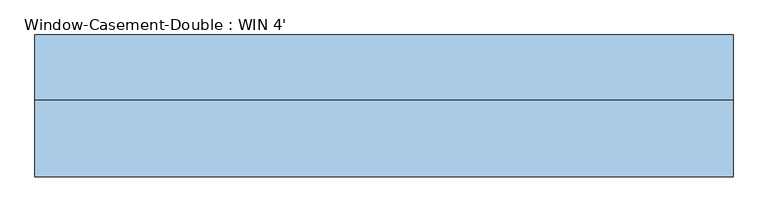
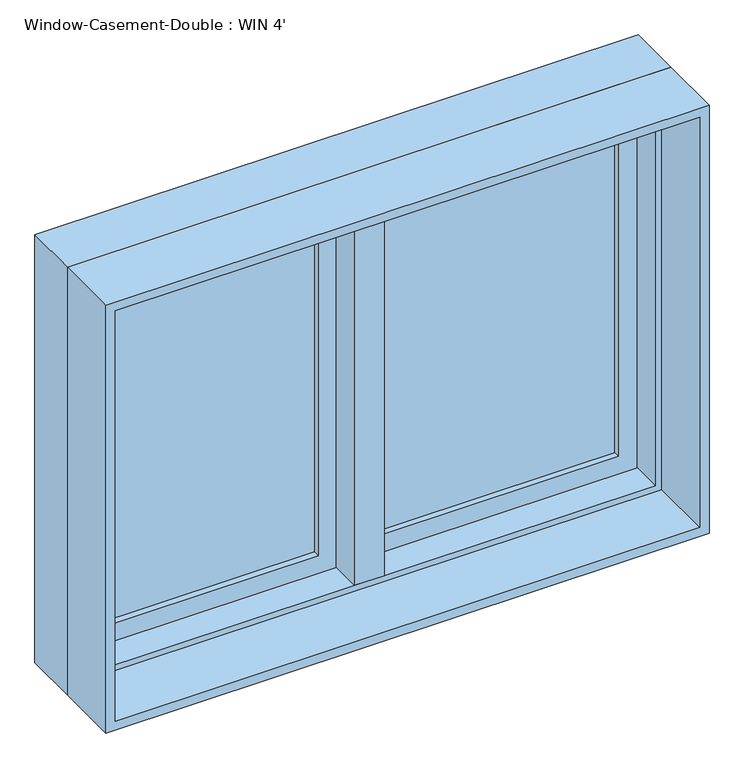
"""IFC4 building model written with IfcOpenShell, lengths in millimetres: window geometry, Window-Casement-Double : WIN 4'."""

from ifc_helpers import new_model, si_unit, frame, origin, place, context, project, spatial, polyline, outline, extrude, faceted_brep, source, transform, mapped, element, save


def window_casement_double_win_4_c19c33cb(model_context):
    return source(origin(), model_context, "Body", "SolidModel", [
        faceted_brep([(9.525, 133.35, 1816.1), (-9.525, 133.35, 1816.1), (-9.525, 82.55, 1816.1), (9.525, 82.55, 1816.1), (9.525, 133.35, 927.1), (9.525, 82.55, 927.1), (-9.525, 82.55, 927.1), (-9.525, 133.35, 927.1), (-9.525, 82.55, 946.15), (-9.525, 82.55, 1797.05), (-30.1625, 82.55, 946.15), (-30.1625, 82.55, 1797.05), (-30.1625, 19.05, 946.15), (-30.1625, 19.05, 1797.05), (30.1625, 19.05, 946.15), (30.1625, 19.05, 1797.05), (30.1625, 82.55, 946.15), (30.1625, 82.55, 1797.05), (9.525, 82.55, 946.15), (9.525, 82.55, 1797.05)], [[[0, 1, 2, 3]], [[4, 5, 6, 7]], [[1, 0, 4, 7]], [[2, 1, 7, 6, 8, 9]], [[9, 8, 10, 11]], [[11, 10, 12, 13]], [[13, 12, 14, 15]], [[15, 14, 16, 17]], [[17, 16, 18, 19]], [[0, 3, 19, 18, 5, 4]], [[18, 8, 6, 5]], [[9, 19, 3, 2]], [[8, 18, 16, 14, 12, 10]], [[19, 9, 11, 13, 15, 17]]]),
        extrude(outline(polyline([(-66.675, 114.3), (-66.675, 107.95), (-539.75, 107.95), (-539.75, 114.3), (-66.675, 114.3)])), frame((0.0, 0.0, 984.25), z_axis=(0.0, 0.0, 1.0), x_axis=(1.0, 0.0, 0.0)), (0.0, 0.0, 1.0), 774.7),
        extrude(outline(polyline([(-539.75, 95.25), (-539.75, 101.6), (-66.675, 101.6), (-66.675, 95.25), (-539.75, 95.25)])), frame((0.0, 0.0, 984.25), z_axis=(0.0, 0.0, 1.0), x_axis=(1.0, 0.0, 0.0)), (0.0, 0.0, 1.0), 774.7),
        extrude(outline(polyline([(539.75, 114.3), (539.75, 107.95), (66.675, 107.95), (66.675, 114.3), (539.75, 114.3)])), frame((0.0, 0.0, 984.25), z_axis=(0.0, 0.0, 1.0), x_axis=(1.0, 0.0, 0.0)), (0.0, 0.0, 1.0), 774.7),
        extrude(outline(polyline([(66.675, 95.25), (66.675, 101.6), (539.75, 101.6), (539.75, 95.25), (66.675, 95.25)])), frame((0.0, 0.0, 984.25), z_axis=(0.0, 0.0, 1.0), x_axis=(1.0, 0.0, 0.0)), (0.0, 0.0, 1.0), 774.7),
        extrude(outline(polyline([(1816.1, -596.9), (927.1, -596.9), (927.1, -9.525), (1816.1, -9.525), (1816.1, -596.9)]), holes=[polyline([(1758.95, -66.675), (984.25, -66.675), (984.25, -539.75), (1758.95, -539.75), (1758.95, -66.675)])]), frame((0.0, 82.55, 0.0), z_axis=(0.0, 1.0, 0.0), x_axis=(0.0, 0.0, 1.0)), (0.0, 0.0, 1.0), 44.45),
        extrude(outline(polyline([(927.1, 596.9), (1816.1, 596.9), (1816.1, 9.525), (927.1, 9.525), (927.1, 596.9)]), holes=[polyline([(984.25, 66.675), (1758.95, 66.675), (1758.95, 539.75), (984.25, 539.75), (984.25, 66.675)])]), frame((0.0, 82.55, 0.0), z_axis=(0.0, 1.0, 0.0), x_axis=(0.0, 0.0, 1.0)), (0.0, 0.0, 1.0), 44.45),
        extrude(outline(polyline([(1828.8, -609.6), (914.4, -609.6), (914.4, 609.6), (1828.8, 609.6), (1828.8, -609.6)]), holes=[polyline([(1809.75, 590.55), (933.45, 590.55), (933.45, -590.55), (1809.75, -590.55), (1809.75, 590.55)])]), frame((0.0, -114.3, 0.0), z_axis=(0.0, 1.0, 0.0), x_axis=(0.0, 0.0, 1.0)), (0.0, 0.0, 1.0), 133.35),
        faceted_brep([(577.85, 82.55, 1797.05), (577.85, 19.05, 1797.05), (-577.85, 19.05, 1797.05), (-577.85, 82.55, 1797.05), (596.9, 133.35, 1816.1), (596.9, 82.55, 1816.1), (-596.9, 82.55, 1816.1), (-596.9, 133.35, 1816.1), (609.6, 19.05, 1828.8), (609.6, 133.35, 1828.8), (-609.6, 133.35, 1828.8), (-609.6, 19.05, 1828.8), (-577.85, 19.05, 946.15), (-577.85, 82.55, 946.15), (-596.9, 82.55, 927.1), (-596.9, 133.35, 927.1), (-609.6, 133.35, 914.4), (-609.6, 19.05, 914.4), (577.85, 19.05, 946.15), (577.85, 82.55, 946.15), (596.9, 82.55, 927.1), (596.9, 133.35, 927.1), (609.6, 133.35, 914.4), (609.6, 19.05, 914.4)], [[[0, 1, 2, 3]], [[4, 5, 6, 7]], [[8, 9, 10, 11]], [[3, 2, 12, 13]], [[7, 6, 14, 15]], [[11, 10, 16, 17]], [[13, 12, 18, 19]], [[15, 14, 20, 21]], [[17, 16, 22, 23]], [[11, 17, 23, 8], [1, 18, 12, 2]], [[19, 18, 1, 0]], [[5, 20, 14, 6], [3, 13, 19, 0]], [[21, 20, 5, 4]], [[23, 22, 9, 8]], [[9, 22, 16, 10], [7, 15, 21, 4]]]),
    ])


if __name__ == "__main__":
    model = new_model("IFC4")
    model_context = context("Model", 3, world=origin())
    ifc_project = project(units=[si_unit("LENGTHUNIT", "METRE", prefix="MILLI")], contexts=[model_context])
    site = spatial("IfcSite", under=ifc_project)
    building = spatial("IfcBuilding", under=site)
    placement = place(None, origin())
    window_casement_double_win_4_shape = window_casement_double_win_4_c19c33cb(model_context)
    element("IfcWindow", 1, ObjectType="Window-Casement-Double : WIN 4'", at=placement, inside=building, context=model_context, shape_type="MappedRepresentation", body=[
        mapped(window_casement_double_win_4_shape, transform((0.0, 0.0, 0.0), x_axis=(1.0, 0.0, 0.0), y_axis=(0.0, 1.0, 0.0), z_axis=(0.0, 0.0, 1.0))),
    ])
    save(model, "model.ifc")

# Revit data of these elements
# Type "Window-Casement-Double : WIN 4'"
#   Type Mark = "18"
#   Fire Rating = "0.5h"
#   Assembly Code = "B2020100"
#   Analytic Construction = "Double glazing - domestic"
#   Frame Extension [instance default] = 0' - 0 1/4"
#   Window Inset [instance default] = 0' - 0"
#   Wall Thickness [instance default] = 0' - 6"
#   Interior Wall Closure [instance default] = 0' - 2 1/4"
#   Half Width = 2' - 0"
#   Visual Light Transmittance = 0.81
#   Thermal Resistance (R) = 1.8146 (h·ft²·°F)/BTU
#   Solar Heat Gain Coefficient = 0.76
#   Rough Width = 4' - 0 1/2"
#   Rough Height = 3' - 0 1/2"
#   Height = 3' - 0"
#   Heat Transfer Coefficient (U) = 0.5511 BTU/(h·ft²·°F)
#   Exterior Wall Closure [instance default] = 0' - 1 1/4"
#   Extension Jamb [instance default] = 0' - 2 1/4"
#   Default Sill Height = 3' - 0"
#   Width = 4' - 0"
#   Muntin Visibility = yes
#   Interior Trim Visibility [instance default] = yes
#   Exterior Trim Visibility [instance default] = yes
#   Extension Jamb Visibility [instance default] = yes
#   Interior Trim Material = Wood - Stained
#   Muntin Pattern = Muntin Pattern_2x2 : Muntin Pattern_2x2
#   Interior Trim = Trim-Window-Interior-Flat : Picture Frame
#   Interior Frame Material = Wood - Stained
#   Glass Panel Material = Glass
#   Exterior Trim Material = Clad - White
#   Exterior Trim = Trim-Window-Exterior-Flat : with Sill
#   Exterior Frame Material = Clad - White
#   Wall Closure = (empty or 0)
# Element 1 (IfcWindow, "Window-Casement-Double : WIN 4'")
#   Wall Thickness = 0' - 9"
#   Extension Jamb = 0' - 5 1/4"
#   Materials on its faces: "Wood - Stained", "Glass", "Clad - White"
# Materials
#   "Wood - Stained": class "Wood", colour RGB 224 178 126, transparency 0, Cost = 0
#   "Glass": class "Glass", colour RGB 0 128 192, transparency 0.75, Description = "Soda Lime Glass", Cost = 0
#   "Clad - White": class "Wood", colour RGB 242 242 238, transparency 0, Cost = 0
